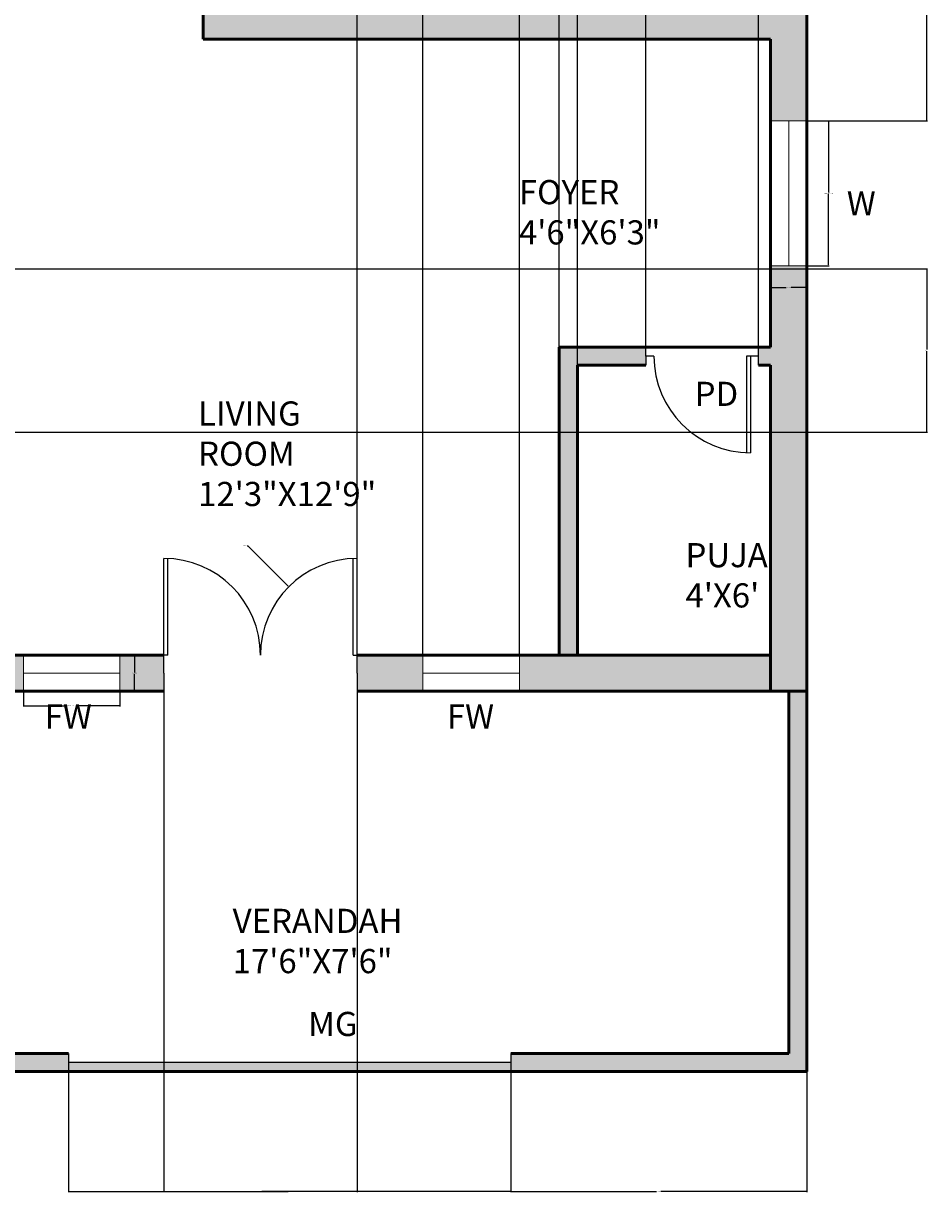
# Model space of a CAD drawing. Units: inches. Extents: x -55 to 413, y -498 to 86.
# Tile 2 of 6: x 188 to 413, y -491 to -201. Entities that reach past the tile are written whole.
import ezdxf

# ---------------------------------------------------------------- set-up
doc = ezdxf.new("R2010")
doc.units = ezdxf.units.IN
doc.header["$MEASUREMENT"] = 0
for name, color, linetype, lineweight in [('A-ANNO-DIMS', 2, 'Continuous', 18), ('A-ANNO-TEXT', 7, 'Continuous', 25), ('A-AREA-IDEN', 7, 'Continuous', 25), ('A-DOOR', 3, 'Continuous', 25), ('A-GLAZ', 4, 'Continuous', 18), ('A-WALL', 7, 'Continuous', 50), ('A-WALL-PATT', 8, 'Continuous', 13)]:
    doc.layers.add(name, color=color, linetype=linetype, lineweight=lineweight)
doc.styles.get("Standard").update_dxf_attribs({"font": 'arial.ttf'})
doc.dimstyles.get("Standard").update_dxf_attribs({"dimtxt": 0.18, "dimasz": 0.18, "dimexe": 0.18, "dimexo": 0.0625, "dimgap": 0.09, "dimtad": 0, "dimtih": 1, "dimtoh": 1, "dimdec": 0, "dimzin": 0, "dimdsep": 46, "dimlunit": 3, "dimtxsty": 'Standard', "dimcen": 0.09, "dimadec": 0, "dimazin": 0, "dimtfac": 1, "dimtdec": 0, "dimtofl": 0, "dimtmove": 0, "dimatfit": 3, "dimfxl": 1, "dimtolj": 1, "dimtzin": 0, "dimarcsym": 0})

# ---------------------------------------------------------------- blocks, each defined once
blk = doc.blocks.new('WIN-24IN')
for p, q in [((24, 9), (0, 9)), ((0, 9), (0, 0)), ((24, 0), (24, 9)), ((0, 4.5), (24, 4.5)), ((0, 0), (24, 0))]:
    blk.add_line(p, q)
blk = doc.blocks.new('WIN-36IN')
for p, q in [((0, 36), (0, 0)), ((9, 36), (0, 36)), ((4.5, 36), (4.5, 0)), ((9, 0), (9, 36)), ((0, 0), (9, 0))]:
    blk.add_line(p, q)
blk = doc.blocks.new('*D13')
at = {"layer": 'A-ANNO-DIMS', "color": 0, "lineweight": -2, "transparency": 16777216}
for p, q in [((188.35, -366.52), (188.35, -370.24)), ((212.35, -366.52), (212.35, -370.24)), ((188.53, -370.06), (199.13, -370.06)), ((212.17, -370.06), (201.57, -370.06))]:
    blk.add_line(p, q, dxfattribs=at)
at = {"layer": 'A-ANNO-DIMS', "color": 0, "transparency": 16777216}
for points in [[(188.53, -370.03), (188.53, -370.09), (188.35, -370.06)], [(212.17, -370.03), (212.17, -370.09), (212.35, -370.06)]]:
    blk.add_solid(points, dxfattribs=at)
at = {"layer": 'Defpoints', "color": 0, "transparency": 16777216}
for p in [(188.35, -366.46), (212.35, -366.46), (212.35, -370.06)]:
    blk.add_point(p, dxfattribs=at)
at = {"layer": 'A-ANNO-DIMS', "color": 0, "transparency": 16777216, "insert": (200.35, -370.06), "char_height": 0.18, "attachment_point": 5}
blk.add_mtext('\\A1;GLAZING 2\'-0" TYP.', dxfattribs=at)
blk = doc.blocks.new('*D14')
at = {"layer": 'A-ANNO-DIMS', "color": 0, "lineweight": -2, "transparency": 16777216}
for p, q in [((212.41, -357.46), (216.13, -357.46)), ((215.95, -357.64), (215.95, -361.78)), ((215.95, -366.28), (215.95, -362.14)), ((212.41, -366.46), (216.13, -366.46))]:
    blk.add_line(p, q, dxfattribs=at)
at = {"layer": 'A-ANNO-DIMS', "color": 0, "transparency": 16777216}
for points in [[(215.92, -357.64), (215.98, -357.64), (215.95, -357.46)], [(215.92, -366.28), (215.98, -366.28), (215.95, -366.46)]]:
    blk.add_solid(points, dxfattribs=at)
at = {"layer": 'Defpoints', "color": 0, "transparency": 16777216}
for p in [(212.35, -357.46), (215.95, -357.46), (212.35, -366.46)]:
    blk.add_point(p, dxfattribs=at)
at = {"layer": 'A-ANNO-DIMS', "color": 0, "transparency": 16777216, "insert": (215.95, -361.96), "char_height": 0.18, "attachment_point": 5}
blk.add_mtext('\\A1;0\'-9" TYP.', dxfattribs=at)
blk = doc.blocks.new('*D15')
at = {"layer": 'A-ANNO-DIMS', "color": 0, "lineweight": -2, "transparency": 16777216}
for p, q in [((383.07, -224.71), (388.58, -224.71)), ((388.4, -224.89), (388.4, -242.53)), ((388.4, -260.53), (388.4, -242.89)), ((383.07, -260.71), (388.58, -260.71))]:
    blk.add_line(p, q, dxfattribs=at)
at = {"layer": 'A-ANNO-DIMS', "color": 0, "transparency": 16777216}
for points in [[(388.37, -224.89), (388.43, -224.89), (388.4, -224.71)], [(388.37, -260.53), (388.43, -260.53), (388.4, -260.71)]]:
    blk.add_solid(points, dxfattribs=at)
at = {"layer": 'Defpoints', "color": 0, "transparency": 16777216}
for p in [(383, -224.71), (388.4, -224.71), (383, -260.71)]:
    blk.add_point(p, dxfattribs=at)
at = {"layer": 'A-ANNO-DIMS', "color": 0, "transparency": 16777216, "insert": (388.4, -242.71), "char_height": 0.18, "attachment_point": 5}
blk.add_mtext('\\A1;WINDOW 3\'-0" TYP.', dxfattribs=at)
blk = doc.blocks.new('*D16')
at = {"layer": 'A-ANNO-DIMS', "color": 0, "lineweight": -2, "transparency": 16777216}
for p, q in [((374, -260.77), (374, -266.29)), ((383, -260.77), (383, -266.29)), ((374.18, -266.11), (377.86, -266.11)), ((382.82, -266.11), (379.14, -266.11))]:
    blk.add_line(p, q, dxfattribs=at)
at = {"layer": 'A-ANNO-DIMS', "color": 0, "transparency": 16777216}
for points in [[(374.18, -266.08), (374.18, -266.14), (374, -266.11)], [(382.82, -266.08), (382.82, -266.14), (383, -266.11)]]:
    blk.add_solid(points, dxfattribs=at)
at = {"layer": 'Defpoints', "color": 0, "transparency": 16777216}
for p in [(374, -260.71), (383, -260.71), (383, -266.11)]:
    blk.add_point(p, dxfattribs=at)
at = {"layer": 'A-ANNO-DIMS', "color": 0, "transparency": 16777216, "insert": (378.5, -266.11), "char_height": 0.18, "attachment_point": 5}
blk.add_mtext('\\A1;0\'-9" TYP.', dxfattribs=at)
blk = doc.blocks.new('*D34')
at = {"layer": 'A-ANNO-DIMS', "color": 0, "lineweight": -2, "transparency": 16777216}
for p, q in [((383.07, -159.01), (412.98, -159.01)), ((412.8, -159.19), (412.8, -191.68)), ((412.8, -224.53), (412.8, -192.04)), ((383.07, -224.71), (412.98, -224.71))]:
    blk.add_line(p, q, dxfattribs=at)
at = {"layer": 'A-ANNO-DIMS', "color": 0, "transparency": 16777216}
for points in [[(412.77, -159.19), (412.83, -159.19), (412.8, -159.01)], [(412.77, -224.53), (412.83, -224.53), (412.8, -224.71)]]:
    blk.add_solid(points, dxfattribs=at)
at = {"layer": 'Defpoints', "color": 0, "transparency": 16777216}
for p in [(383, -159.01), (383, -224.71), (412.8, -224.71)]:
    blk.add_point(p, dxfattribs=at)
at = {"layer": 'A-ANNO-DIMS', "color": 0, "transparency": 16777216, "insert": (412.8, -191.86), "char_height": 0.18, "attachment_point": 5}
blk.add_mtext('\\A1;5\'-5 1/2"', dxfattribs=at)
blk = doc.blocks.new('*D35')
at = {"layer": 'A-ANNO-DIMS', "color": 0, "lineweight": -2, "transparency": 16777216}
for p, q in [((164.07, -261.46), (412.98, -261.46)), ((412.8, -261.64), (412.8, -281.58)), ((412.8, -301.89), (412.8, -281.95)), ((164.07, -302.07), (412.98, -302.07))]:
    blk.add_line(p, q, dxfattribs=at)
at = {"layer": 'A-ANNO-DIMS', "color": 0, "transparency": 16777216}
for points in [[(412.77, -261.64), (412.83, -261.64), (412.8, -261.46)], [(412.77, -301.89), (412.83, -301.89), (412.8, -302.07)]]:
    blk.add_solid(points, dxfattribs=at)
at = {"layer": 'Defpoints', "color": 0, "transparency": 16777216}
for p in [(164, -261.46), (412.8, -261.46), (164, -302.07)]:
    blk.add_point(p, dxfattribs=at)
at = {"layer": 'A-ANNO-DIMS', "color": 0, "transparency": 16777216, "insert": (412.8, -281.76), "char_height": 0.18, "attachment_point": 5}
blk.add_mtext('\\A1;3\'-4 1/2"', dxfattribs=at)
blk = doc.blocks.new('*D36')
at = {"layer": 'A-ANNO-DIMS', "color": 0, "lineweight": -2, "transparency": 16777216}
for p, q in [((343, -280.9), (343, 47.52)), ((343.18, 47.34), (356.67, 47.34)), ((370.82, 47.34), (357.33, 47.34)), ((371, -280.9), (371, 47.52))]:
    blk.add_line(p, q, dxfattribs=at)
at = {"layer": 'A-ANNO-DIMS', "color": 0, "transparency": 16777216}
for points in [[(343.18, 47.37), (343.18, 47.31), (343, 47.34)], [(370.82, 47.37), (370.82, 47.31), (371, 47.34)]]:
    blk.add_solid(points, dxfattribs=at)
at = {"layer": 'Defpoints', "color": 0, "transparency": 16777216}
for p in [(371, 47.34), (343, -280.96), (371, -280.96)]:
    blk.add_point(p, dxfattribs=at)
at = {"layer": 'A-ANNO-DIMS', "color": 0, "transparency": 16777216, "insert": (357, 47.34), "char_height": 0.18, "attachment_point": 5}
blk.add_mtext('\\A1;2\'-4"', dxfattribs=at)
blk = doc.blocks.new('*D37')
at = {"layer": 'A-ANNO-DIMS', "color": 0, "lineweight": -2, "transparency": 16777216}
for p, q in [((321.5, -280.9), (321.5, 47.52)), ((321.68, 47.34), (323.21, 47.34)), ((325.82, 47.34), (324.29, 47.34)), ((326, -285.4), (326, 47.52))]:
    blk.add_line(p, q, dxfattribs=at)
at = {"layer": 'A-ANNO-DIMS', "color": 0, "transparency": 16777216}
for points in [[(321.68, 47.37), (321.68, 47.31), (321.5, 47.34)], [(325.82, 47.37), (325.82, 47.31), (326, 47.34)]]:
    blk.add_solid(points, dxfattribs=at)
at = {"layer": 'Defpoints', "color": 0, "transparency": 16777216}
for p in [(326, 47.34), (321.5, -280.96), (326, -285.46)]:
    blk.add_point(p, dxfattribs=at)
at = {"layer": 'A-ANNO-DIMS', "color": 0, "transparency": 16777216, "insert": (323.75, 47.34), "char_height": 0.18, "attachment_point": 5}
blk.add_mtext('\\A1;0\'-4 1/2"', dxfattribs=at)
blk = doc.blocks.new('*D38')
at = {"layer": 'A-ANNO-DIMS', "color": 0, "lineweight": -2, "transparency": 16777216}
for p, q in [((223.25, -366.52), (223.25, -490.94)), ((271.25, -366.52), (271.25, -490.94)), ((223.43, -490.76), (246.92, -490.76)), ((271.07, -490.76), (247.59, -490.76))]:
    blk.add_line(p, q, dxfattribs=at)
at = {"layer": 'A-ANNO-DIMS', "color": 0, "transparency": 16777216}
for points in [[(223.43, -490.73), (223.43, -490.79), (223.25, -490.76)], [(271.07, -490.73), (271.07, -490.79), (271.25, -490.76)]]:
    blk.add_solid(points, dxfattribs=at)
at = {"layer": 'Defpoints', "color": 0, "transparency": 16777216}
for p in [(223.25, -366.46), (271.25, -366.46), (271.25, -490.76)]:
    blk.add_point(p, dxfattribs=at)
at = {"layer": 'A-ANNO-DIMS', "color": 0, "transparency": 16777216, "insert": (247.25, -490.76), "char_height": 0.18, "attachment_point": 5}
blk.add_mtext('\\A1;4\'-0"', dxfattribs=at)
blk = doc.blocks.new('*D39')
at = {"layer": 'A-ANNO-DIMS', "color": 0, "lineweight": -2, "transparency": 16777216}
for p, q in [((271.25, -357.4), (271.25, 47.52)), ((271.43, 47.34), (278.91, 47.34)), ((287.45, 47.34), (279.97, 47.34)), ((287.63, -357.4), (287.63, 47.52))]:
    blk.add_line(p, q, dxfattribs=at)
at = {"layer": 'A-ANNO-DIMS', "color": 0, "transparency": 16777216}
for points in [[(271.43, 47.37), (271.43, 47.31), (271.25, 47.34)], [(287.45, 47.37), (287.45, 47.31), (287.63, 47.34)]]:
    blk.add_solid(points, dxfattribs=at)
at = {"layer": 'Defpoints', "color": 0, "transparency": 16777216}
for p in [(287.63, 47.34), (271.25, -357.46), (287.63, -357.46)]:
    blk.add_point(p, dxfattribs=at)
at = {"layer": 'A-ANNO-DIMS', "color": 0, "transparency": 16777216, "insert": (279.44, 47.34), "char_height": 0.18, "attachment_point": 5}
blk.add_mtext('\\A1;1\'-4 1/2"', dxfattribs=at)
blk = doc.blocks.new('*D42')
at = {"layer": 'A-ANNO-DIMS', "color": 0, "lineweight": -2, "transparency": 16777216}
for p, q in [((311.63, -357.4), (311.63, 47.52)), ((311.81, 47.34), (316.17, 47.34)), ((321.32, 47.34), (316.97, 47.34)), ((321.5, -357.4), (321.5, 47.52))]:
    blk.add_line(p, q, dxfattribs=at)
at = {"layer": 'A-ANNO-DIMS', "color": 0, "transparency": 16777216}
for points in [[(311.81, 47.37), (311.81, 47.31), (311.63, 47.34)], [(321.32, 47.37), (321.32, 47.31), (321.5, 47.34)]]:
    blk.add_solid(points, dxfattribs=at)
at = {"layer": 'Defpoints', "color": 0, "transparency": 16777216}
for p in [(321.5, 47.34), (311.63, -357.46), (321.5, -357.46)]:
    blk.add_point(p, dxfattribs=at)
at = {"layer": 'A-ANNO-DIMS', "color": 0, "transparency": 16777216, "insert": (316.57, 47.34), "char_height": 0.18, "attachment_point": 5}
blk.add_mtext('\\A1;0\'-10"', dxfattribs=at)
blk = doc.blocks.new('*D46')
at = {"layer": 'A-ANNO-DIMS', "color": 0, "lineweight": -2, "transparency": 16777216}
for p, q in [((199.52, -461.02), (199.52, -490.94)), ((309.45, -461.02), (309.45, -490.94)), ((199.7, -490.76), (254.16, -490.76)), ((309.27, -490.76), (254.81, -490.76))]:
    blk.add_line(p, q, dxfattribs=at)
at = {"layer": 'A-ANNO-DIMS', "color": 0, "transparency": 16777216}
for points in [[(199.7, -490.73), (199.7, -490.79), (199.52, -490.76)], [(309.27, -490.73), (309.27, -490.79), (309.45, -490.76)]]:
    blk.add_solid(points, dxfattribs=at)
at = {"layer": 'Defpoints', "color": 0, "transparency": 16777216}
for p in [(199.52, -460.96), (309.45, -460.96), (309.45, -490.76)]:
    blk.add_point(p, dxfattribs=at)
at = {"layer": 'A-ANNO-DIMS', "color": 0, "transparency": 16777216, "insert": (254.48, -490.76), "char_height": 0.18, "attachment_point": 5}
blk.add_mtext('\\A1;9\'-2"', dxfattribs=at)
blk = doc.blocks.new('*D47')
at = {"layer": 'A-ANNO-DIMS', "color": 0, "lineweight": -2, "transparency": 16777216}
for p, q in [((309.45, -461.02), (309.45, -490.94)), ((383, -461.02), (383, -490.94)), ((309.63, -490.76), (345.69, -490.76)), ((382.82, -490.76), (346.76, -490.76))]:
    blk.add_line(p, q, dxfattribs=at)
at = {"layer": 'A-ANNO-DIMS', "color": 0, "transparency": 16777216}
for points in [[(309.63, -490.73), (309.63, -490.79), (309.45, -490.76)], [(382.82, -490.73), (382.82, -490.79), (383, -490.76)]]:
    blk.add_solid(points, dxfattribs=at)
at = {"layer": 'Defpoints', "color": 0, "transparency": 16777216}
for p in [(309.45, -460.96), (383, -460.96), (383, -490.76)]:
    blk.add_point(p, dxfattribs=at)
at = {"layer": 'A-ANNO-DIMS', "color": 0, "transparency": 16777216, "insert": (346.23, -490.76), "char_height": 0.18, "attachment_point": 5}
blk.add_mtext('\\A1;6\'-1 1/2"', dxfattribs=at)
blk = doc.blocks.new('*D50')
at = {"layer": 'A-ANNO-DIMS', "color": 0, "lineweight": -2, "transparency": 16777216}
for p, q in [((243.92, -330.31), (244.1, -330.31)), ((244.1, -330.31), (254.15, -340.36)), ((271.16, -357.46), (271.34, -357.46)), ((271.25, -357.55), (271.25, -357.37))]:
    blk.add_line(p, q, dxfattribs=at)
at = {"layer": 'A-ANNO-DIMS', "color": 0, "transparency": 16777216}
blk.add_solid([(254.18, -340.34), (254.13, -340.38), (254.28, -340.49)], dxfattribs=at)
at = {"layer": 'Defpoints', "color": 0, "transparency": 16777216}
for p in [(254.28, -340.49), (271.25, -357.46)]:
    blk.add_point(p, dxfattribs=at)
at = {"layer": 'A-ANNO-DIMS', "color": 0, "transparency": 16777216, "insert": (243.31, -330.31), "char_height": 0.18, "attachment_point": 5}
blk.add_mtext('\\A1;5X R2\'-0"', dxfattribs=at)

msp = doc.modelspace()

# ---------------------------------------------------------------- hatches: boundary and pattern name
at = {"layer": 'A-WALL-PATT'}
h = msp.add_hatch(color=256, dxfattribs=at)
h.dxf.hatch_style = 1
h.paths.add_polyline_path([(97.55, 17.54), (23, 17.54), (23, -94.08), (32, -94.08), (32, 8.54), (97.55, 8.54)])
h.paths.add_polyline_path([(191, 17.54), (157.55, 17.54), (157.55, 8.54), (164, 8.54), (164, -80.46), (168.5, -80.46), (173, -80.46), (173, 8.54), (191, 8.54)])
h.paths.add_polyline_path([(312.03, 17.54), (215, 17.54), (215, 8.54), (233, 8.54), (233, -111.46), (173, -111.46), (173, -108.46), (164, -108.46), (164, -164.46), (168.5, -164.46), (173, -164.46), (173, -120.46), (233, -120.46), (233, -164.46), (237.5, -164.46), (242, -164.46), (242, 8.54), (312.03, 8.54)])
h.paths.add_polyline_path([(383, 17.54), (372.03, 17.54), (372.03, 8.54), (374, 8.54), (374, -99.01), (383, -99.01)])
h.paths.add_polyline_path([(383, -159.01), (374, -159.01), (374, -195.46), (242, -195.46), (242, -192.46), (233, -192.46), (233, -204.46), (374, -204.46), (374, -224.71), (383, -224.71)])
h.paths.add_polyline_path([(173, -192.46), (164, -192.46), (164, -195.46), (32, -195.46), (32, -154.08), (23, -154.08), (23, -213.4), (32, -213.4), (32, -204.46), (164, -204.46), (164, -221.46), (168.5, -221.46), (173, -221.46)])
h.paths.add_polyline_path([(173, -249.46), (164, -249.46), (164, -252.46), (32, -252.46), (32, -237.4), (23, -237.4), (23, -273.22), (32, -273.22), (32, -261.46), (164, -261.46), (173, -261.46)])
h.paths.add_polyline_path([(32, -309.22), (23, -309.22), (23, -456.46), (23, -460.96), (199.52, -460.96), (199.52, -456.46), (32, -456.46), (32, -366.46), (97.71, -366.46), (97.71, -357.46), (32, -357.46)])
h.paths.add_polyline_path([(188.35, -357.46), (173, -357.46), (173, -302.07), (164, -302.07), (164, -357.46), (157.71, -357.46), (157.71, -366.46), (188.35, -366.46)])
h.paths.add_polyline_path([(223.25, -357.46), (212.35, -357.46), (212.35, -366.46), (223.25, -366.46), (223.25, -361.96)])
h.paths.add_polyline_path([(287.63, -357.46), (271.25, -357.46), (271.25, -361.96), (271.25, -366.46), (287.63, -366.46)])
h.paths.add_polyline_path([(374, -357.46), (311.63, -357.46), (311.63, -366.46), (374, -366.46)])
h.paths.add_polyline_path([(383, -456.46), (383, -366.46), (378.5, -366.46), (378.5, -456.46), (309.45, -456.46), (309.45, -460.96), (383, -460.96)])
h.paths.add_polyline_path([(309.45, -458.71), (199.52, -458.71), (199.52, -460.96), (309.45, -460.96)])
h.paths.add_polyline_path([(383, -260.71), (374, -260.71), (374, -280.96), (371, -280.96), (371, -285.46), (374, -285.46), (374, -366.46), (383, -366.46)])
h.paths.add_polyline_path([(343, -283.21), (343, -280.96), (321.5, -280.96), (321.5, -357.46), (326, -357.46), (326, -285.46), (343, -285.46)])

# ---------------------------------------------------------------- linework, layer by layer
at = {"layer": 'A-DOOR'}
for p, q in [((343, -283.21), (343, -280.96)), ((371, -285.46), (371, -280.96)), ((345, -283.21), (343, -283.21)), ((343, -283.21), (343, -285.46)), ((368, -283.21), (368, -307.21)), ((369, -283.21), (368, -283.21)), ((371, -283.21), (369, -283.21)), ((369, -283.21), (369, -307.21)), ((223.25, -357.46), (223.25, -333.46)), ((224.25, -357.46), (224.25, -333.46)), ((270.25, -357.46), (270.25, -333.46)), ((271.25, -357.46), (271.25, -333.46)), ((223.25, -361.96), (223.25, -357.46)), ((224.25, -357.46), (223.25, -357.46)), ((270.25, -357.46), (271.25, -357.46)), ((271.25, -361.96), (271.25, -357.46)), ((223.25, -361.96), (223.25, -366.46)), ((271.25, -361.96), (271.25, -366.46)), ((199.52, -456.46), (199.52, -460.96)), ((309.45, -458.71), (199.52, -458.71)), ((309.45, -456.46), (309.45, -460.96))]:
    msp.add_line(p, q, dxfattribs=at)
for centre, start, end in [((369, -283.21), 180, 270), ((223.25, -357.46), 0, 90), ((271.25, -357.46), 90, 180)]:
    msp.add_arc(centre, 24, start, end, dxfattribs=at)
at = {"layer": 'A-WALL'}
for p, q in [((383, 17.54), (383, -456.46)), ((233, -120.46), (233, -204.46)), ((233, -204.46), (374, -204.46)), ((374, -204.46), (374, -280.96)), ((321.5, -280.96), (374, -280.96)), ((321.5, -280.96), (321.5, -357.46)), ((326, -285.46), (326, -357.46)), ((326, -285.46), (343, -285.46)), ((371, -285.46), (374, -285.46)), ((374, -285.46), (374, -366.46)), ((173, -357.46), (223.25, -357.46)), ((173, -357.46), (223.25, -357.46)), ((271.25, -357.46), (374, -357.46)), ((271.25, -357.46), (321.5, -357.46)), ((32, -366.46), (223.25, -366.46)), ((271.25, -366.46), (383, -366.46)), ((378.5, -366.46), (378.5, -456.46)), ((32, -456.46), (199.52, -456.46)), ((309.45, -456.46), (378.5, -456.46)), ((383, -460.96), (383, -456.46)), ((23, -460.96), (383, -460.96))]:
    msp.add_line(p, q, dxfattribs=at)

# ---------------------------------------------------------------- block references
at = {"layer": 'A-GLAZ'}
for name, p in [('WIN-36IN', (374, -260.71)), ('WIN-24IN', (188.35, -366.46)), ('WIN-24IN', (287.63, -366.46))]:
    msp.add_blockref(name, p, dxfattribs=at)

# ---------------------------------------------------------------- texts
at = {"layer": 'A-ANNO-TEXT', "char_height": 6, "attachment_point": 1}
for s, insert in [('W', (392.94, -242.2)), ('PD', (355.14, -289.56)), ('FW', (193.65, -369.72)), ('FW', (293.58, -369.72)), ('MG', (259.1, -446.12))]:
    msp.add_mtext(s, dxfattribs=dict(at, insert=insert))
at = {"layer": 'A-AREA-IDEN', "char_height": 6, "attachment_point": 1}
for s, insert in [('FOYER\\P4\'6"X6\'3"', (311.47, -239.44)), ('LIVING\\PROOM\\P12\'3"X12\'9"', (231.77, -294.44)), ("PUJA\\P4'X6'", (352.86, -329.64)), ('VERANDAH\\P17\'6"X7\'6"', (240.35, -420.51))]:
    msp.add_mtext(s, dxfattribs=dict(at, insert=insert))

# ---------------------------------------------------------------- dimensions: what is measured, and where the dimension line sits
at = {"layer": 'A-ANNO-DIMS'}
for base, p1, p2, picture, middle in [((287.63, 47.34), (271.25, -357.46), (287.63, -357.46), '*D39', (279.44, 47.34)), ((321.5, 47.34), (311.63, -357.46), (321.5, -357.46), '*D42', (316.57, 47.34)), ((326, 47.34), (321.5, -280.96), (326, -285.46), '*D37', (323.75, 47.34)), ((371, 47.34), (343, -280.96), (371, -280.96), '*D36', (357, 47.34)), ((271.25, -490.76), (223.25, -366.46), (271.25, -366.46), '*D38', (247.25, -490.76)), ((309.45, -490.76), (199.52, -460.96), (309.45, -460.96), '*D46', (254.48, -490.76)), ((383.0027, -490.7603), (309.4476, -460.9603), (383.0027, -460.9603), '*D47', (346.2251, -490.7603))]:
    dim = msp.add_linear_dim(base=base, p1=p1, p2=p2, dimstyle='Standard', override={"dimdec": 1, "dimlfac": 1, "dimrnd": 0, "dimzin": 1, "dimdsep": 46, "dimlunit": 4, "dimfrac": 2}, dxfattribs=at)
    dim.commit()
    dim.dimension.update_dxf_attribs({"geometry": picture, "text_midpoint": middle})
for base, p1, p2, picture, middle in [((412.8, -224.71), (383, -159.01), (383, -224.71), '*D34', (412.8, -191.86)), ((412.8, -261.46), (164, -302.07), (164, -261.46), '*D35', (412.8, -281.76))]:
    dim = msp.add_linear_dim(base=base, p1=p1, p2=p2, angle=90, dimstyle='Standard', override={"dimdec": 1, "dimlfac": 1, "dimrnd": 0, "dimzin": 1, "dimdsep": 46, "dimlunit": 4, "dimfrac": 2}, dxfattribs=at)
    dim.commit()
    dim.dimension.update_dxf_attribs({"geometry": picture, "text_midpoint": middle})
for base, p1, p2, text, picture, middle in [((388.4, -224.71), (383, -260.71), (383, -224.71), 'WINDOW <> TYP.', '*D15', (388.4, -242.71)), ((215.95, -357.46), (212.35, -366.46), (212.35, -357.46), '<> TYP.', '*D14', (215.95, -361.96))]:
    dim = msp.add_linear_dim(base=base, p1=p1, p2=p2, angle=90, text=text, dimstyle='Standard', override={"dimdec": 1, "dimlfac": 1, "dimrnd": 0, "dimzin": 1, "dimdsep": 46, "dimlunit": 4, "dimfrac": 2}, dxfattribs=at)
    dim.commit()
    dim.dimension.update_dxf_attribs({"geometry": picture, "text_midpoint": middle})
for base, p1, p2, text, picture, middle in [((383, -266.11), (374, -260.71), (383, -260.71), '<> TYP.', '*D16', (378.5, -266.11)), ((212.35, -370.06), (188.35, -366.46), (212.35, -366.46), 'GLAZING <> TYP.', '*D13', (200.35, -370.06))]:
    dim = msp.add_linear_dim(base=base, p1=p1, p2=p2, text=text, dimstyle='Standard', override={"dimdec": 1, "dimlfac": 1, "dimrnd": 0, "dimzin": 1, "dimdsep": 46, "dimlunit": 4, "dimfrac": 2}, dxfattribs=at)
    dim.commit()
    dim.dimension.update_dxf_attribs({"geometry": picture, "text_midpoint": middle})
dim = msp.add_radius_dim(center=(271.25, -357.46), mpoint=(254.28, -340.49), text='5X <>', dimstyle='Standard', override={"dimdec": 1, "dimlfac": 1, "dimrnd": 0, "dimzin": 1, "dimdsep": 46, "dimlunit": 4, "dimfrac": 2}, dxfattribs=at)
dim.commit()
dim.dimension.update_dxf_attribs({"geometry": '*D50', "text_midpoint": (243.31, -330.31), "dimtype": 164})

doc.saveas('drawing.dxf')
